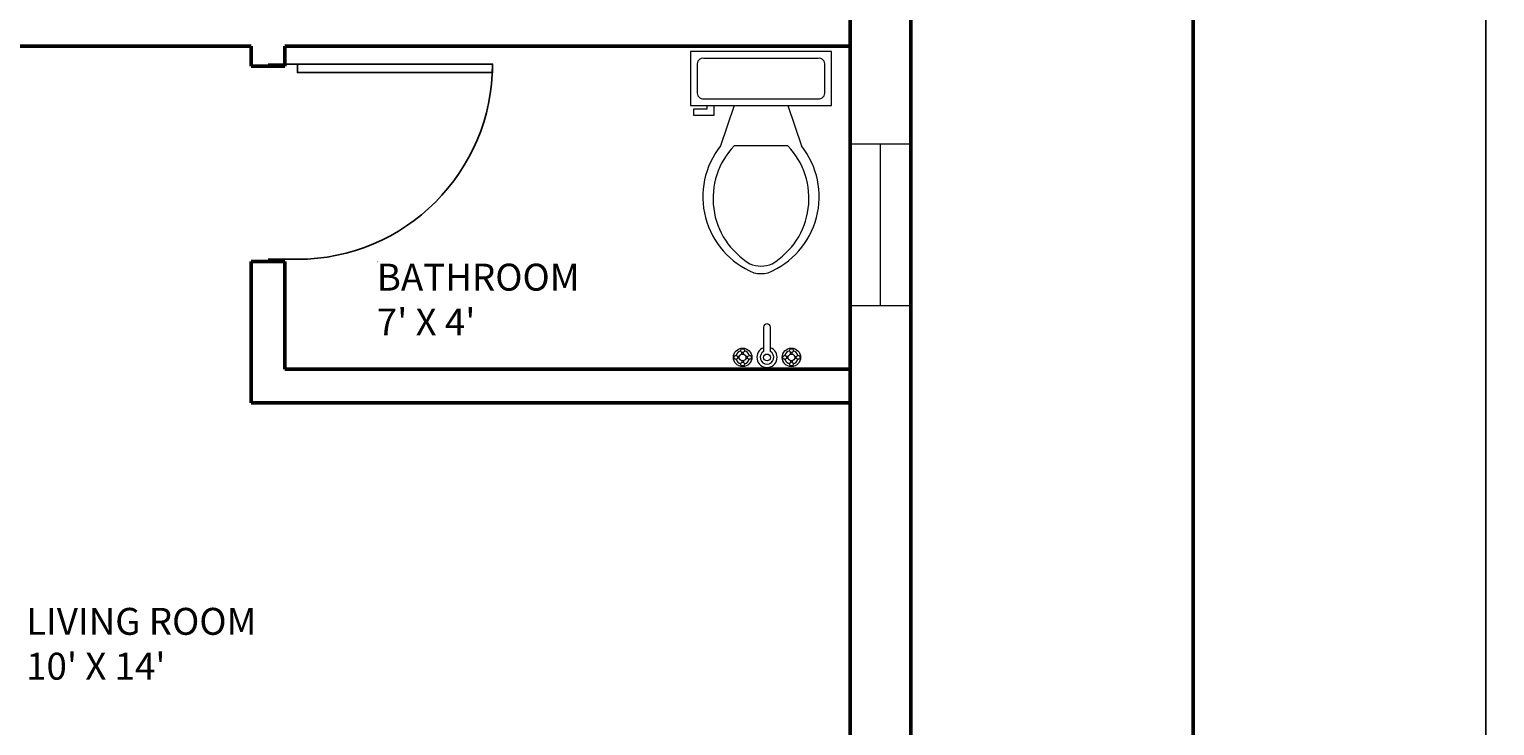
# Model space of a CAD drawing. Units: inches. Extents: x 3506 to 3958, y 1553 to 2506.
# Tile 8 of 16: x 3739 to 3957, y 1899 to 2003. Entities that reach past the tile are written whole.
import ezdxf

# ---------------------------------------------------------------- set-up
doc = ezdxf.new("R2010")
doc.units = ezdxf.units.IN
doc.header["$MEASUREMENT"] = 0
for name, color, linetype, lineweight in [('A-ANNO-DIMS', 2, 'Continuous', 18), ('A-AREA-IDEN', 7, 'Continuous', 18), ('A-WALL', 7, 'Continuous', 50), ('bathroom', 90, 'Continuous', 18), ('doors', 40, 'Continuous', 25), ('window', 30, 'Continuous', 20)]:
    doc.layers.add(name, color=color, linetype=linetype, lineweight=lineweight)
doc.layers.add('A-WALL-PATT', color=251, linetype='Continuous', lineweight=13, true_color=0x636466)
doc.styles.get("Standard").update_dxf_attribs({"font": 'arial.ttf'})
doc.dimstyles.get("Standard").update_dxf_attribs({"dimtxt": 1.18, "dimasz": 0.68, "dimexe": 0.18, "dimexo": 0.0625, "dimgap": 0.09, "dimtad": 0, "dimtih": 1, "dimtoh": 1, "dimdec": 1, "dimzin": 0, "dimdsep": 46, "dimlunit": 3, "dimtxsty": 'Standard', "dimcen": 0.09, "dimadec": 0, "dimazin": 0, "dimtfac": 1, "dimtdec": 1, "dimtofl": 0, "dimtmove": 0, "dimatfit": 3, "dimfxl": 1, "dimtolj": 1, "dimtzin": 0, "dimarcsym": 0})

# ---------------------------------------------------------------- blocks, each defined once
blk = doc.blocks.new('*U10')
for p, q in [((0, 0), (0, -6)), ((40, 0), (40, -6))]:
    blk.add_line(p, q)
blk.add_lwpolyline([(0, 0), (0, 40), (1.75, 40), (1.75, 0)], close=True)
blk.add_arc((0, 0), 40, 0, 90)
blk = doc.blocks.new('Faucet - Bathroom top')
for p, q in [((-4.107, 0.125), (-4.375, 0.125)), ((-3.75, 0.4788), (-3.75, 0.75)), ((-3.5, 0.482), (-3.5, 0.75)), ((-3.1461, 0.125), (-2.875, 0.125)), ((3.143, 0.125), (2.875, 0.125)), ((3.5, 0.4788), (3.5, 0.75)), ((3.75, 0.482), (3.75, 0.75)), ((4.1039, 0.125), (4.375, 0.125)), ((-4.1039, -0.125), (-4.375, -0.125)), ((-3.75, -0.4821), (-3.75, -0.75)), ((-3.5, -0.4789), (-3.5, -0.75)), ((-3.143, -0.125), (-2.875, -0.125)), ((-0.5, -0.8639), (-0.5, -4.5)), ((0.5, -4.5), (0.5, -0.8631)), ((3.1461, -0.125), (2.875, -0.125)), ((3.5, -0.4821), (3.5, -0.75)), ((3.75, -0.4789), (3.75, -0.75)), ((4.107, -0.125), (4.375, -0.125))]:
    blk.add_line(p, q)
for centre, radius in [((-3.625, 0), 1.375), ((-4.625, 0), 0.2795), ((-3.625, 0), 0.5), ((-3.625, 1), 0.2795), ((-2.625, 0), 0.2795), ((0, 0), 0.5), ((3.625, 0), 1.375), ((2.625, 0), 0.2795), ((3.625, 0), 0.5), ((3.625, 1), 0.2795), ((4.625, 0), 0.2795), ((-3.625, -1), 0.2795), ((3.625, -1), 0.2795)]:
    blk.add_circle(centre, radius)
for centre, radius, start, end in [((-3.625, 0), 1, 105.2407, 164.2093), ((-3.625, 0), 1, 16.44125, 74.07887), ((0, 0), 1.5, 289.6514, 250.3603), ((0, 0), 1, 300.3431, 239.7554), ((3.625, 0), 1, 106.12, 164.0884), ((3.625, 0), 1, 16.23422, 73.90469), ((-3.625, 0), 1, 196.2342, 253.9047), ((-3.625, 0), 1, 286.12, 344.0884), ((3.625, 0), 1, 196.4413, 254.0789), ((3.625, 0), 1, 285.2407, 344.2093), ((0, -4.5), 0.5, 180, 0)]:
    blk.add_arc(centre, radius, start, end)
blk = doc.blocks.new('Toilet - top')
for p, q in [((9.5, -6), (9.5, -2)), ((-10, -8.5), (-8, -8.5)), ((-10, -9.5), (-10, -8.5)), ((-8, -8.5), (-8, -8)), ((-7, -8), (-7, -9.5)), ((-4, -8), (-6, -14)), ((4, -8), (6, -14)), ((-7, -9.5), (-10, -9.5)), ((4, -14), (-4, -14))]:
    blk.add_line(p, q)
blk.add_lwpolyline([(10.5, -8), (10.5, 0), (-10.5, 0), (-10.5, -8)], close=True)
for points in [[(-9.5, -2), (-9.5, -6)], [(8.5, -1), (-8.5, -1)], [(-8.5, -7), (8.5, -7)]]:
    blk.add_lwpolyline(points)
for centre, radius, start, end in [((-8.62, -1.88), 0.884, 81.8699, 188.1301), ((8.62, -1.88), 0.884, 351.8699, 98.1301), ((-8.62, -6.12), 0.884, 171.8699, 278.1301), ((8.62, -6.12), 0.884, 261.8699, 8.1301), ((3.52, -21.58), 12.17, 141.4691, 247.9714), ((4.2, -21.82), 11.33, 136.3677, 238.9468), ((-3.52, -21.58), 12.17, 292.0284, 38.5307), ((-4.2, -21.82), 11.33, 301.053, 43.6321), ((0, -27.88), 4, 245.7318, 294.2682), ((0, -29), 4, 254.8605, 285.1395)]:
    blk.add_arc(centre, radius, start, end)
blk = doc.blocks.new('WIN-24IN-9IN-WALL')
for p, q in [((0, 0), (0, 9)), ((0, 9), (24, 9)), ((24, 9), (24, 0)), ((0, 0), (0, 4.5)), ((0, 4.5), (24, 4.5)), ((24, 0), (0, 0))]:
    blk.add_line(p, q)
blk = doc.blocks.new('*D39')
at = {"layer": 'A-ANNO-DIMS', "color": 0, "lineweight": -2, "transparency": 16777216}
for p, q in [((3911.79, 2461.39), (3955.36, 2461.39)), ((3955.18, 2460.71), (3955.18, 2030.09)), ((3955.18, 1598.07), (3955.18, 2028.7)), ((3911.79, 1597.39), (3955.36, 1597.39))]:
    blk.add_line(p, q, dxfattribs=at)
at = {"layer": 'A-ANNO-DIMS', "color": 0, "transparency": 16777216}
for points in [[(3955.07, 2460.71), (3955.29, 2460.71), (3955.18, 2461.39)], [(3955.07, 1598.07), (3955.29, 1598.07), (3955.18, 1597.39)]]:
    blk.add_solid(points, dxfattribs=at)
at = {"layer": 'Defpoints', "color": 0, "transparency": 16777216}
for p in [(3911.73, 2461.39), (3955.18, 2461.39), (3911.73, 1597.39)]:
    blk.add_point(p, dxfattribs=at)
at = {"layer": 'A-ANNO-DIMS', "color": 0, "transparency": 16777216, "insert": (3955.18, 2029.39), "char_height": 1.18, "attachment_point": 5}
blk.add_mtext('\\A1;864', dxfattribs=at)

msp = doc.modelspace()

# ---------------------------------------------------------------- hatches: boundary and pattern name
at = {"layer": 'A-WALL-PATT'}
h = msp.add_hatch(dxfattribs=at)
h.set_pattern_fill('ANSI31', color=256)
h.paths.add_polyline_path([(3911.7302, 2461.3942), (3551.7302, 2461.3942), (3551.7302, 2152.516), (3560.7302, 2152.516), (3560.7302, 2116.516), (3551.7302, 2116.516), (3551.7302, 1920.5711), (3556.2302, 1920.5711), (3560.7302, 1920.5711), (3560.7302, 2000.3942), (3692.7302, 2000.3942), (3692.7302, 1997.3942), (3697.7302, 1997.3942), (3697.7302, 2000.3942), (3771.7302, 2000.3942), (3771.7302, 1997.3942), (3776.7302, 1997.3942), (3776.7302, 1997.7206), (3778.5802, 1997.7206), (3807.5802, 1997.7206), (3807.5802, 1996.4519), (3778.5802, 1996.4519), (3778.5802, 1997.7206), (3776.7302, 1997.7206), (3776.7302, 1997.3942), (3771.7302, 1997.3942), (3771.7302, 2000.3942), (3697.7302, 2000.3942), (3697.7302, 1997.3942), (3692.7302, 1997.3942), (3689.8302, 1997.3942), (3689.8302, 1995.8192), (3653.8302, 1995.8192), (3653.8302, 1997.3942), (3689.8302, 1997.3942), (3692.7302, 1997.3942), (3692.7302, 2000.3942), (3560.7302, 2000.3942), (3560.7302, 1920.5711), (3551.7302, 1920.5711), (3551.7302, 1884.5711), (3551.7302, 1597.3942), (3911.7302, 1597.3942)], flags=17)
h.paths.add_polyline_path([(3596.7302, 2005.3942), (3596.7302, 2057.3035, -0.38730371), (3569.1778, 2085), (3569.15, 2085), (3569.15, 2086.2688), (3598.15, 2086.2688), (3598.15, 2085), (3569.1778, 2085, 0.38730371), (3596.7302, 2057.3035), (3596.7302, 2057.3942), (3601.7302, 2057.3942), (3601.7302, 2055.3942), (3630.7302, 2055.3942), (3630.7302, 2034.3942), (3694.7302, 2034.3942), (3694.7302, 2053.3942), (3699.7302, 2053.3942), (3699.7302, 2005.3942), (3860.7302, 2005.3942), (3860.7302, 2173.3942), (3771.7302, 2173.3942), (3771.7302, 2194.3942), (3776.7302, 2194.3942), (3776.7302, 2178.3942), (3860.7302, 2178.3942), (3860.7302, 2231.3942), (3601.7302, 2231.3942), (3601.7302, 2241.426), (3596.7302, 2241.426), (3596.7302, 2231.3942), (3560.7302, 2231.3942), (3560.7302, 2315.3942), (3596.7302, 2315.3942), (3596.7302, 2312.3942), (3601.7302, 2312.3942), (3601.7302, 2315.3942), (3697.7302, 2315.3942), (3697.7302, 2413.3942), (3692.7302, 2413.3942), (3692.7302, 2320.3942), (3560.7302, 2320.3942), (3560.7302, 2452.3942), (3692.7302, 2452.3942), (3692.7302, 2449.3942), (3697.7302, 2449.3942), (3697.7302, 2452.3942), (3771.7302, 2452.3942), (3771.7302, 2449.3942), (3776.7302, 2449.3942), (3776.7302, 2452.3942), (3860.7302, 2452.3942), (3860.7302, 2437.2075), (3865.2302, 2437.2075), (3865.2302, 2413.2075), (3860.7302, 2413.2075), (3860.7302, 2367.6976), (3865.2302, 2367.6976), (3869.7302, 2367.6976), (3869.7302, 2319.6976), (3860.7302, 2319.6976), (3860.7302, 2211.6248), (3869.7302, 2211.6248), (3869.7302, 2187.6248), (3860.7302, 2187.6248), (3860.7302, 2138.4346), (3865.2302, 2138.4346), (3869.7302, 2138.4346), (3869.7302, 2090.4346), (3860.7302, 2090.4346), (3860.7302, 1985.8449), (3869.7302, 1985.8449), (3869.7302, 1961.8449), (3860.7302, 1961.8449), (3860.7302, 1897.0756), (3865.2302, 1897.0756), (3869.7302, 1897.0756), (3869.7302, 1849.0756), (3860.7302, 1849.0756), (3860.7302, 1847.8112), (3860.7302, 1779.3942), (3596.7302, 1779.3942), (3596.7302, 1831.3942), (3601.7302, 1831.3942), (3601.7302, 1828.3942), (3630.7302, 1828.3942), (3630.7302, 1808.3942), (3691.7302, 1808.3942), (3691.7302, 1815.3942), (3696.7302, 1815.3942), (3696.7302, 1779.3942), (3860.7302, 1779.3942), (3860.7302, 1947.3942), (3771.7302, 1947.3942), (3771.7302, 1968.3942), (3776.7302, 1968.3942), (3776.7302, 1952.3942), (3860.7302, 1952.3942), (3860.7302, 2005.3942)], flags=0)
h.paths.add_polyline_path([(3596.7302, 2038.8546), (3601.7302, 2038.8546), (3601.7302, 2014.8546), (3596.7302, 2014.8546)], flags=0)
h.paths.add_polyline_path([(3564.1688, 2107), (3564.1688, 2167), (3644.1688, 2167), (3644.1688, 2107)], flags=0)
h.paths.add_polyline_path([(3607.0972, 2052.0208), (3620.8472, 2052.0208, -0.41421356), (3621.9931, 2050.875), (3621.9931, 2025.6667, -0.41421356), (3620.8472, 2024.5208), (3607.0972, 2024.5208, -0.41421356), (3605.9514, 2025.6667), (3605.9514, 2050.875, -0.41421356)], flags=0)
h.paths.add_polyline_path([(3578.5688, 2115), (3565.3688, 2115), (3565.3688, 2135.8), (3578.5688, 2135.8), (3578.5688, 2138.2), (3565.3688, 2138.2), (3565.3688, 2159), (3580.5688, 2159), (3580.5688, 2153.8), (3593.7688, 2167), (3593.7688, 2151.8), (3578.5688, 2151.8)], flags=0)
h.paths.add_polyline_path([(3610.9167, 2050.875), (3620.0833, 2050.875, -0.41421356), (3620.8472, 2050.1111), (3620.8472, 2039.6076, -0.41421356), (3620.0833, 2038.8438), (3610.9167, 2038.8438, -0.41421356), (3610.1528, 2039.6076), (3610.1528, 2050.1111, -0.41421356)], flags=0)
h.paths.add_polyline_path([(3610.9167, 2037.6979), (3620.0833, 2037.6979, -0.41421356), (3620.8472, 2036.934), (3620.8472, 2026.4306, -0.41421356), (3620.0833, 2025.6667), (3610.9167, 2025.6667, -0.41421356), (3610.1528, 2026.4306), (3610.1528, 2036.934, -0.41421356)], flags=0)
h.paths.add_polyline_path([(3616.2639, 2044.7639, -1), (3614.7361, 2044.7639, -1)], flags=0)
h.paths.add_polyline_path([(3615.8819, 2044.7639, -1), (3615.1181, 2044.7639, -1)], flags=0)
h.paths.add_polyline_path([(3616.2639, 2031.7778, -1), (3614.7361, 2031.7778, -1)], flags=0)
h.paths.add_polyline_path([(3615.8819, 2031.7778, -1), (3615.1181, 2031.7778, -1)], flags=0)
h.paths.add_polyline_path([(3609.7539, 2021.7868), (3626.9586, 2021.7868), (3626.9586, 2008.8833), (3609.7539, 2008.8833)], flags=0)
h.paths.add_polyline_path([(3610.4708, 2021.07), (3621.2237, 2021.07), (3621.2237, 2009.6002), (3610.4708, 2009.6002)], flags=0)
h.paths.add_polyline_path([(3611.5461, 2019.9947), (3620.1484, 2019.9947), (3620.1484, 2010.6755), (3611.5461, 2010.6755)], flags=0)
h.paths.add_polyline_path([(3621.9405, 2021.07), (3626.2417, 2021.07), (3626.2417, 2009.6002), (3621.9405, 2009.6002)], flags=0)
h.paths.add_polyline_path([(3622.6574, 2020.3531), (3625.5248, 2020.3531), (3625.5248, 2017.4857), (3622.6574, 2017.4857)], flags=0)
h.paths.add_polyline_path([(3622.6574, 2016.7688), (3625.5248, 2016.7688), (3625.5248, 2010.317), (3622.6574, 2010.317)], flags=0)
h.paths.add_polyline_path([(3624.808, 2016.0519), (3624.808, 2013.9013), (3624.0911, 2013.9013), (3624.0911, 2013.1845), (3623.3743, 2013.1845), (3623.3743, 2013.9013), (3623.3743, 2016.0519)], flags=0)
h.paths.add_polyline_path([(3623.0158, 2012.8261), (3625.1664, 2012.8261), (3625.1664, 2012.1092), (3623.0158, 2012.1092)], flags=0)
h.paths.add_polyline_path([(3623.0158, 2011.7508), (3625.1664, 2011.7508), (3625.1664, 2011.0339), (3623.0158, 2011.0339)], flags=0)
h.paths.add_polyline_path([(3650.0591, 2031.8202), (3674.0368, 2031.8202), (3674.0368, 2012.638), (3669.2413, 2012.638), (3669.2413, 2011.8388), (3672.4383, 2011.8388), (3672.4383, 2011.0395), (3651.6576, 2011.0395), (3651.6576, 2011.8388), (3654.8546, 2011.8388), (3654.8546, 2012.638), (3650.0591, 2012.638)], flags=0)
h.paths.add_polyline_path([(3658.0517, 2024.6269, -1), (3651.6576, 2024.6269, -1)], flags=0)
h.paths.add_polyline_path([(3657.2524, 2024.6269, -1), (3652.4569, 2024.6269, -1)], flags=0)
h.paths.add_polyline_path([(3656.4532, 2024.6269, -1), (3653.2561, 2024.6269, -1)], flags=0)
h.paths.add_polyline_path([(3655.6539, 2024.6269, -1), (3654.0554, 2024.6269, -1)], flags=0)
h.paths.add_polyline_path([(3657.2524, 2017.4336, -1), (3652.4569, 2017.4336, -1)], flags=0)
h.paths.add_polyline_path([(3656.4532, 2017.4336, -1), (3653.2561, 2017.4336, -1)], flags=0)
h.paths.add_polyline_path([(3655.6539, 2017.4336, -1), (3654.0554, 2017.4336, -1)], flags=0)
h.paths.add_polyline_path([(3659.6502, 2027.8239), (3664.4457, 2027.8239), (3664.4457, 2015.0358), (3659.6502, 2015.0358)], flags=0)
h.paths.add_polyline_path([(3663.6465, 2027.0247), (3663.6465, 2015.8351), (3660.4494, 2015.8351), (3660.4494, 2027.0247)], flags=0)
h.paths.add_polyline_path([(3562.6688, 1945.5), (3642.6688, 1945.5), (3642.6688, 1885.5), (3562.6688, 1885.5)], flags=0)
h.paths.add_polyline_path([(3671.6391, 2024.6269, -1), (3666.8435, 2024.6269, -1)], flags=0)
h.paths.add_polyline_path([(3670.8398, 2024.6269, -1), (3667.6428, 2024.6269, -1)], flags=0)
h.paths.add_polyline_path([(3672.4383, 2017.4336, -1), (3666.0443, 2017.4336, -1)], flags=0)
h.paths.add_polyline_path([(3670.0405, 2024.6269, -1), (3668.442, 2024.6269, -1)], flags=0)
h.paths.add_polyline_path([(3671.6391, 2017.4336, -1), (3666.8435, 2017.4336, -1)], flags=0)
h.paths.add_polyline_path([(3670.8398, 2017.4336, -1), (3667.6428, 2017.4336, -1)], flags=0)
h.paths.add_polyline_path([(3592.2688, 1945.5), (3592.2688, 1930.3), (3577.0688, 1930.3), (3577.0688, 1893.5), (3563.8688, 1893.5), (3563.8688, 1914.3), (3577.0688, 1914.3), (3577.0688, 1916.7), (3563.8688, 1916.7), (3563.8688, 1937.5), (3579.0688, 1937.5), (3579.0688, 1932.3)], flags=0)
h.paths.add_polyline_path([(3670.0405, 2017.4336, -1), (3668.442, 2017.4336, -1)], flags=0)
h.paths.add_polyline_path([(3596.7302, 2283.3942), (3601.7302, 2283.3942), (3601.7302, 2265.426), (3599.2302, 2265.426), (3599.2302, 2241.426), (3596.7302, 2241.426), (3596.7302, 2265.426)], flags=0)
h.paths.add_polyline_path([(3596.7302, 1810.7006), (3601.7302, 1810.7006), (3601.7302, 1786.7006), (3596.7302, 1786.7006)], flags=0)
h.paths.add_polyline_path([(3560.7302, 1770.3942), (3738.7302, 1770.3942), (3738.7302, 1746.3942), (3738.7302, 1722.3942), (3748.7302, 1722.3942), (3748.7302, 1674.3942), (3560.7302, 1674.3942)], flags=0)
h.paths.add_polyline_path([(3728.7302, 1746.3942), (3728.7302, 1756.0642), (3738.7302, 1746.3942), (3728.7302, 1738.1582), (3728.7302, 1698.3942), (3591.2519, 1698.3942), (3591.2519, 1746.3942)], flags=0)
h.paths.add_polyline_path([(3771.7302, 2399.3942), (3771.7302, 2420.3942), (3776.7302, 2420.3942), (3776.7302, 2404.3942), (3776.7302, 2399.3942)], flags=0)
h.paths.add_polyline_path([(3911.7302, 2461.3942), (3551.7302, 2461.3942), (3551.7302, 2152.516), (3560.7302, 2152.516), (3560.7302, 2116.516), (3551.7302, 2116.516), (3551.7302, 1920.5711), (3560.7302, 1920.5711), (3560.7302, 2000.3942), (3692.7302, 2000.3942), (3692.7302, 1997.3942), (3697.7302, 1997.3942), (3697.7302, 2000.3942), (3771.7302, 2000.3942), (3771.7302, 1997.3942), (3776.7302, 1997.3942), (3776.7302, 1997.7206), (3778.5802, 1997.7206), (3807.5802, 1997.7206), (3807.5802, 1996.4519), (3778.5802, 1996.4519), (3778.5802, 1997.7206), (3776.7302, 1997.7206), (3776.7302, 1997.3942), (3771.7302, 1997.3942), (3771.7302, 2000.3942), (3697.7302, 2000.3942), (3697.7302, 1997.3942), (3692.7302, 1997.3942), (3689.8302, 1997.3942), (3689.8302, 1995.8192), (3653.8302, 1995.8192), (3653.8302, 1997.3942), (3689.8302, 1997.3942), (3692.7302, 1997.3942), (3692.7302, 2000.3942), (3560.7302, 2000.3942), (3560.7302, 1920.5711), (3551.7302, 1920.5711), (3551.7302, 1597.3942), (3911.7302, 1597.3942)], flags=17)

# ---------------------------------------------------------------- linework, layer by layer
at = {"layer": 'A-WALL'}
for p, q in [((3860.7302, 2015.4906), (3860.7302, 1838.7087)), ((3869.7302, 2015.4906), (3869.7302, 1838.7087)), ((3697.7302, 2000.3942), (3771.7302, 2000.3942)), ((3771.7302, 2000.3942), (3771.7302, 1997.3942)), ((3771.7302, 2000.3942), (3771.7302, 1997.3942)), ((3776.7302, 2000.3942), (3776.7302, 1997.3942)), ((3776.7302, 2000.3942), (3860.7302, 2000.3942)), ((3771.7302, 1997.3942), (3776.7302, 1997.3942)), ((3771.7302, 1968.3942), (3776.7302, 1968.3942)), ((3771.7302, 1968.3942), (3771.7302, 1947.3942)), ((3776.7302, 1968.3942), (3776.7302, 1952.3942)), ((3776.7302, 1952.3942), (3860.7302, 1952.3942)), ((3771.7302, 1947.3942), (3860.7302, 1947.3942))]:
    msp.add_line(p, q, dxfattribs=at)
msp.add_lwpolyline([(3551.7302, 2461.3942), (3911.7302, 2461.3942), (3911.7302, 1597.3942), (3551.7302, 1597.3942)], close=True, dxfattribs=at)

# ---------------------------------------------------------------- block references
at = {"layer": 'bathroom'}
msp.add_blockref('Toilet - top', (3847.4804, 1999.5805), dxfattribs=at)
at = {"layer": 'bathroom', "rotation": 180}
msp.add_blockref('Faucet - Bathroom top', (3848.375, 1954.1369), dxfattribs=at)
at = {"layer": 'doors', "xscale": 0.725, "yscale": 0.725, "zscale": 0.725, "rotation": 270}
msp.add_blockref('*U10', (3778.5802, 1997.7206), dxfattribs=at)
at = {"layer": 'window', "extrusion": (0, 0, -1), "zscale": -1, "rotation": 90.00000000000333}
msp.add_blockref('WIN-24IN-9IN-WALL', (-3860.7301, 1961.8447), dxfattribs=at)

# ---------------------------------------------------------------- texts
at = {"layer": 'A-AREA-IDEN', "attachment_point": 1}
for s, width, insert, char_height in [('4"\\P{\\H20x;BATHROOM\\P7\' X 4\'}', 25.775469, (3790.3788, 1968.3942), 0.2), ("LIVING ROOM\\P10' X 14'", 79.631666, (3738.2651, 1916.9071), 4)]:
    msp.add_mtext_dynamic_manual_height_columns(s, width=width, gutter_width=1, heights=[0], dxfattribs=dict(at, insert=insert, char_height=char_height))

# ---------------------------------------------------------------- dimensions: what is measured, and where the dimension line sits
at = {"layer": 'A-ANNO-DIMS'}
dim = msp.add_linear_dim(base=(3955.1802, 2461.3942), p1=(3911.7302, 1597.3942), p2=(3911.7302, 2461.3942), angle=90, dimstyle='Standard', override={"dimdec": 0, "dimlfac": 1, "dimrnd": 0, "dimzin": 0, "dimdsep": 46, "dimlunit": 2}, dxfattribs=at)
dim.commit()
dim.dimension.update_dxf_attribs({"geometry": '*D39', "text_midpoint": (3955.1802, 2029.3942)})

doc.saveas('drawing.dxf')
